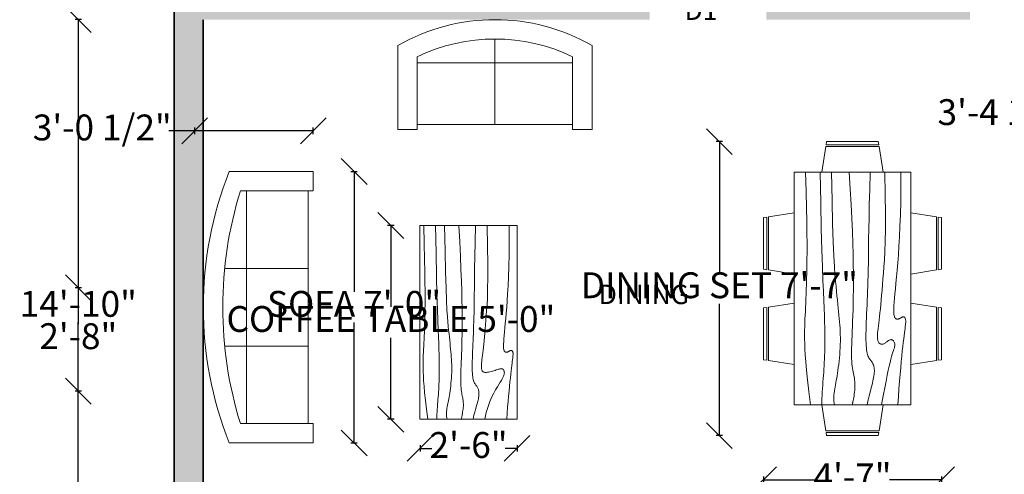
# Model space of a CAD drawing. Units: inches. Extents: x 2530 to 3100, y 543 to 1175.
# Tile 3 of 5: x 2578 to 2883, y 804 to 944. Entities that reach past the tile are written whole.
import ezdxf

# ---------------------------------------------------------------- set-up
doc = ezdxf.new("R2010")
doc.units = ezdxf.units.IN
for name, color, linetype, lineweight in [('A-ANNO-DIMS', 2, 'Continuous', 18), ('A-ANNO-TEXT', 7, 'Continuous', 18), ('A-AREA-IDEN', 7, 'Continuous', 18), ('A-FURN', 8, 'Continuous', 18), ('A-WALL', 7, 'Continuous', 35), ('A-WALL-PATT', 30, 'Continuous', 13)]:
    doc.layers.add(name, color=color, linetype=linetype, lineweight=lineweight)
doc.styles.get("Standard").update_dxf_attribs({"font": 'arial.ttf'})
doc.dimstyles.new('ISO-25', dxfattribs={"dimtxt": 8, "dimasz": 8, "dimexe": 1, "dimexo": 1, "dimtad": 0, "dimtih": 1, "dimtoh": 1, "dimlunit": 3, "dimtxsty": 'Standard', "dimblk": 'OBLIQUE', "dimcen": 2.5, "dimadec": 0, "dimazin": 0, "dimtfac": 1, "dimtmove": 0, "dimatfit": 3, "dimfxl": 1, "dimfxlon": 1, "dimarcsym": 0})

# ---------------------------------------------------------------- blocks, each defined once
blk = doc.blocks.new('Sofa - Roundback 7 ft.')
for p, q in [((-12.00002, -32.4421), (-12.00003, -6.5971)), ((11.99997, -32.4421), (11.99998, -6.5971)), ((-36.000027, -34), (-36.000027, -11.4696)), ((35.99998, -34), (35.99998, -11.4696)), ((-35.999844, -13.3819), (35.9998, -13.3819)), ((-36.000027, -32.4421), (35.99998, -32.4421))]:
    blk.add_line(p, q)
for points in [[(-36.000027, -34), (-42.000027, -34), (-42.000027, -8)], [(41.99998, -8), (41.99998, -34), (35.99998, -34)]]:
    blk.add_lwpolyline(points)
for centre, radius, start, end in [((0, -114.25), 114.25, 68.43141, 111.5686), ((-0.00001, -127.1968), 121.1968, 72.72033, 107.2797)]:
    blk.add_arc(centre, radius, start, end)
blk = doc.blocks.new('Sofa - Roundback Loveseat 5 ft.')
for p, q in [((0, -32.44198), (0, -5.99998)), ((-24, -33.99998), (-24, -11.46958)), ((24.00004, -33.99998), (24.00004, -11.46958)), ((-23.9998, -13.38178), (23.99986, -13.38178)), ((-24, -32.44198), (24.00004, -32.44198))]:
    blk.add_line(p, q)
for points in [[(-24, -33.99998), (-30, -33.99998), (-30, -7.99998)], [(30.00004, -7.99998), (30.00004, -33.99998), (24.00004, -33.99998)]]:
    blk.add_lwpolyline(points)
for centre, radius, start, end in [((0, -60.24998), 60.24998, 60.13715, 119.8628), ((0, -61.38438), 55.38444, 64.32083, 115.6792)]:
    blk.add_arc(centre, radius, start, end)
blk = doc.blocks.new('Dining Set - 36 x 72 in.')
for p, q in [((-22, 27.5), (-22.1562, 26.50042)), ((-22, 27.5), (-6, 27.5)), ((-5.8437, 26.49966), (-6, 27.5)), ((6, 27.5), (5.8438, 26.50042)), ((6, 27.5), (22, 27.5)), ((22.1563, 26.49966), (22, 27.5)), ((-22.2343, 26.00059), (-23.4847, 17.99762)), ((-22.2304, 26), (-5.7608, 26)), ((-5.8416, 26.5), (-22.1534, 26.5)), ((-4.5152, 17.99762), (-5.7655, 25.99926)), ((5.7657, 26.00059), (4.5153, 17.99762)), ((5.7696, 26), (22.2392, 26)), ((22.1584, 26.5), (5.8466, 26.5)), ((23.4848, 17.99762), (22.2345, 25.99926)), ((36, 18), (-36, 18)), ((-36, 18), (-36, -18)), ((36, -18), (36, 18)), ((-44.0006, 8.23428), (-35.9976, 9.48474)), ((44.0006, 8.23428), (35.9976, 9.48474)), ((-45.5, 8), (-44.5004, 8.15617)), ((-45.5, 8), (-45.5, -8)), ((-44.5, -8.15843), (-44.5, 8.15338)), ((-44, 8.23041), (-44, -8.23915)), ((44, 8.23041), (44, -8.23915)), ((44.5, -8.15843), (44.5, 8.15338)), ((45.5, 8), (44.5005, 8.15617)), ((45.5, 8), (45.5, -8)), ((-44.4997, -8.15631), (-45.5, -8)), ((-35.9976, -9.48476), (-43.9993, -8.2345)), ((35.9976, -9.48476), (43.9993, -8.2345)), ((44.4997, -8.15631), (45.5, -8)), ((-36, -18), (36, -18)), ((-22.2343, -26.0006), (-23.4847, -17.99762)), ((-4.5152, -17.99762), (-5.7655, -25.99928)), ((5.7657, -26.0006), (4.5153, -17.99762)), ((23.4848, -17.99762), (22.2345, -25.99928)), ((-22.2304, -26), (-5.7608, -26)), ((-22, -27.5), (-22.1562, -26.50044)), ((-5.8416, -26.5), (-22.1534, -26.5)), ((-5.8437, -26.49967), (-6, -27.5)), ((5.7696, -26), (22.2392, -26)), ((6, -27.5), (5.8438, -26.50044)), ((22.1584, -26.5), (5.8466, -26.5)), ((22.1563, -26.49967), (22, -27.5)), ((-22, -27.5), (-6, -27.5)), ((6, -27.5), (22, -27.5))]:
    blk.add_line(p, q)
for points in [[(-36, 15), (-31.1772, 14.97754), (-26.8079, 14.91406), (-22.8538, 14.81543), (-19.276, 14.6875), (-16.0362, 14.53613), (-13.0957, 14.36718), (-10.4159, 14.18652), (-7.9583, 14), (-5.6904, 13.81315), (-3.6035, 13.63021), (-1.6954, 13.45508), (0.0365, 13.29166), (1.5945, 13.14388), (2.9811, 13.01562), (4.1988, 12.9108), (5.25, 12.83333), (6.1393, 12.78613), (6.8802, 12.76823), (7.4883, 12.77767), (7.9792, 12.8125), (8.3685, 12.87077), (8.6719, 12.95052), (8.9049, 13.0498), (9.0833, 13.16666), (9.2205, 13.29899), (9.3216, 13.44401), (9.3895, 13.59879), (9.4271, 13.76041), (9.4373, 13.92594), (9.4232, 14.09245), (9.3875, 14.257), (9.3333, 14.41666), (9.2638, 14.56917), (9.1836, 14.71484), (9.0975, 14.85465), (9.0104, 14.98958), (8.9272, 15.1206), (8.8529, 15.2487), (8.7922, 15.37483), (8.75, 15.5), (8.7305, 15.62467), (8.7344, 15.74739), (8.7617, 15.86621), (8.8125, 15.97916), (8.8867, 16.08431), (8.9844, 16.17968), (9.1055, 16.26334), (9.25, 16.33333), (9.4189, 16.38802), (9.6172, 16.42708), (9.8506, 16.45052), (10.125, 16.45833), (10.4463, 16.45052), (10.8203, 16.42708), (11.2529, 16.38802), (11.75, 16.33333), (12.3184, 16.26318), (12.9694, 16.17838), (13.7151, 16.07991), (14.5677, 15.96875), (15.5395, 15.84586), (16.6426, 15.71224), (17.8893, 15.56884), (19.2917, 15.41666), (20.859, 15.25667), (22.5879, 15.08984), (24.4721, 14.91715), (26.5052, 14.73958), (28.6809, 14.5581), (30.9929, 14.3737), (33.4347, 14.18733), (36, 14)], [(-36, 10), (-28.9766, 10.14274), (-23.1725, 10.20442), (-18.4241, 10.19775), (-14.5677, 10.13541), (-11.4399, 10.03011), (-8.877, 9.89453), (-6.7154, 9.74137), (-4.7917, 9.58333), (-2.9698, 9.43082), (-1.2246, 9.28515), (0.4415, 9.14534), (2.026, 9.01041), (3.5266, 8.87939), (4.9408, 8.7513), (6.266, 8.62516), (7.5, 8.5), (8.6411, 8.37549), (9.6914, 8.2539), (10.6538, 8.13818), (11.5312, 8.03125), (12.3267, 7.93603), (13.043, 7.85547), (13.6831, 7.79248), (14.25, 7.75), (14.7471, 7.7303), (15.1797, 7.73307), (15.5537, 7.75732), (15.875, 7.80208), (16.1494, 7.86637), (16.3828, 7.94922), (16.5811, 8.04964), (16.75, 8.16666), (16.8944, 8.29915), (17.0143, 8.44531), (17.1089, 8.60319), (17.1771, 8.77083), (17.218, 8.94629), (17.2305, 9.1276), (17.2137, 9.31282), (17.1667, 9.5), (17.0895, 9.6875), (16.987, 9.875), (16.8649, 10.0625), (16.7292, 10.25), (16.5856, 10.4375), (16.4401, 10.625), (16.2985, 10.8125), (16.1667, 11), (16.05, 11.18733), (15.9518, 11.3737), (15.8752, 11.5581), (15.8229, 11.73958), (15.798, 11.91715), (15.8034, 12.08984), (15.842, 12.25667), (15.9167, 12.41666), (16.0295, 12.56836), (16.1784, 12.70833), (16.3605, 12.83268), (16.5729, 12.9375), (16.8127, 13.01888), (17.0768, 13.07291), (17.3625, 13.0957), (17.6667, 13.08333), (17.9894, 13.03312), (18.3418, 12.94726), (18.7382, 12.82918), (19.1927, 12.68229), (19.7195, 12.51001), (20.3327, 12.31575), (21.0465, 12.10294), (21.875, 11.875), (22.8357, 11.63354), (23.959, 11.37304), (25.2786, 11.08618), (26.8282, 10.76562), (28.6414, 10.40405), (30.752, 9.99414), (33.1936, 9.52856), (36, 9)], [(-36, 5.5), (-30.7157, 5.3348), (-26.069, 5.20963), (-21.9946, 5.11767), (-18.4271, 5.05208), (-15.3009, 5.00602), (-12.5508, 4.97265), (-10.1112, 4.94515), (-7.9167, 4.91666), (-5.909, 4.88167), (-4.0586, 4.83984), (-2.3429, 4.79215), (-0.7396, 4.73958), (0.7739, 4.6831), (2.22, 4.6237), (3.6213, 4.56233), (5, 4.5), (6.373, 4.43782), (7.7344, 4.3776), (9.0723, 4.32129), (10.375, 4.27083), (11.6309, 4.22819), (12.8281, 4.19531), (13.9551, 4.17415), (15, 4.16666), (15.954, 4.17448), (16.819, 4.19791), (17.6001, 4.23698), (18.3021, 4.29166), (18.9299, 4.36198), (19.4883, 4.44791), (19.9823, 4.54948), (20.4167, 4.66666), (20.7969, 4.79899), (21.1302, 4.94401), (21.4245, 5.09879), (21.6875, 5.26041), (21.9271, 5.42594), (22.1511, 5.59245), (22.3672, 5.757), (22.5834, 5.91666), (22.8065, 6.06868), (23.0404, 6.21093), (23.2879, 6.34147), (23.5521, 6.45833), (23.8358, 6.55957), (24.142, 6.64323), (24.4735, 6.70735), (24.8334, 6.75), (25.2235, 6.76969), (25.642, 6.76692), (26.0858, 6.74267), (26.5521, 6.69791), (27.0379, 6.63362), (27.5404, 6.55078), (28.0565, 6.45036), (28.5834, 6.33333), (29.1242, 6.19987), (29.7071, 6.04687), (30.3661, 5.87044), (31.1354, 5.66666), (32.0493, 5.43164), (33.142, 5.16146), (34.4475, 4.85221), (36, 4.5)], [(-36, -1), (-30.7915, -0.6591), (-26.0195, -0.38216), (-21.6519, -0.16284), (-17.6563, 0.00521), (-14.0005, 0.12833), (-10.6523, 0.21289), (-7.5796, 0.26522), (-4.75, 0.29166), (-2.134, 0.29793), (0.2878, 0.28711), (2.5317, 0.26163), (4.6146, 0.22396), (6.5529, 0.17651), (8.3633, 0.12174), (10.0623, 0.06209), (11.6667, 0), (13.1899, -0.06201), (14.6341, -0.1211), (15.9982, -0.17432), (17.2813, -0.21875), (18.4823, -0.25147), (19.6003, -0.26953), (20.6343, -0.27002), (21.5834, -0.25), (22.4481, -0.20768), (23.2357, -0.14584), (23.9549, -0.06836), (24.6146, 0.02083), (25.2235, 0.11784), (25.7904, 0.21875), (26.3241, 0.31966), (26.8334, 0.41666), (27.3265, 0.50618), (27.8099, 0.58593), (28.2894, 0.65397), (28.7709, 0.70833), (29.2601, 0.74707), (29.763, 0.76823), (30.2855, 0.76985), (30.8334, 0.75), (31.4088, 0.70784), (31.9994, 0.64713), (32.589, 0.57275), (33.1615, 0.48958), (33.7008, 0.4025), (34.1908, 0.3164), (34.6153, 0.23616), (34.9584, 0.16666), (35.2099, 0.11165), (35.3848, 0.07031), (35.504, 0.04069), (35.5886, 0.02083), (35.6594, 0.00879), (35.7377, 0.0026), (35.8442, 0.00032), (36, 0)], [(-36, -6.5), (-27.1843, -6.31267), (-20.084, -6.1263), (-14.469, -5.9419), (-10.1094, -5.76042), (-6.7752, -5.58285), (-4.2363, -5.41016), (-2.2629, -5.24333), (-0.625, -5.08334), (0.8708, -4.93099), (2.2715, -4.78646), (3.5872, -4.64974), (4.8281, -4.52084), (6.0046, -4.39974), (7.127, -4.28646), (8.2053, -4.18099), (9.25, -4.08334), (10.2705, -3.99382), (11.2734, -3.91407), (12.2647, -3.84603), (13.25, -3.79167), (14.2354, -3.75293), (15.2266, -3.73177), (16.2295, -3.73015), (17.25, -3.75), (18.2912, -3.79248), (19.3451, -3.85547), (20.4009, -3.93604), (21.4479, -4.03125), (22.4754, -4.13819), (23.4727, -4.25391), (24.4289, -4.37549), (25.3334, -4.5), (26.1785, -4.62492), (26.9694, -4.74935), (27.7145, -4.87281), (28.4219, -4.99479), (29.1, -5.11483), (29.7572, -5.23242), (30.4016, -5.34709), (31.0417, -5.45834), (31.6837, -5.56437), (32.3262, -5.65821), (32.9658, -5.73153), (33.599, -5.77604), (34.2224, -5.78345), (34.8327, -5.74545), (35.4264, -5.65373), (36, -5.5)], [(-36, -10), (-26.4022, -9.81299), (-18.4675, -9.62891), (-11.9839, -9.45069), (-6.7396, -9.28125), (-2.5226, -9.12354), (0.8789, -8.98047), (3.6769, -8.85498), (6.0833, -8.75), (8.2767, -8.66765), (10.3021, -8.60677), (12.1712, -8.56543), (13.8958, -8.54167), (15.4876, -8.53353), (16.9583, -8.53907), (18.3197, -8.55632), (19.5834, -8.58334), (20.7616, -8.61841), (21.8685, -8.66081), (22.9188, -8.71004), (23.9271, -8.76563), (24.9081, -8.82707), (25.8763, -8.89388), (26.8465, -8.96558), (27.8334, -9.04167), (28.8474, -9.12118), (29.8828, -9.20117), (30.93, -9.27824), (31.9792, -9.34896), (33.0205, -9.40991), (34.0443, -9.45768), (35.0407, -9.48885), (36, -9.5)], [(-36, -14.5), (-30.0881, -14.33513), (-25.0332, -14.21224), (-20.7312, -14.12647), (-17.0781, -14.07292), (-13.97, -14.04671), (-11.3027, -14.04297), (-8.9724, -14.05681), (-6.875, -14.08334), (-4.9224, -14.11833), (-3.0905, -14.16016), (-1.3709, -14.20785), (0.2448, -14.26042), (1.7647, -14.3169), (3.1973, -14.3763), (4.5507, -14.43767), (5.8333, -14.5), (7.0554, -14.5621), (8.235, -14.62175), (9.3922, -14.67652), (10.5469, -14.72396), (11.7192, -14.76164), (12.929, -14.78711), (14.1965, -14.79794), (15.5417, -14.79167), (16.9933, -14.76424), (18.6152, -14.70508), (20.4804, -14.60197), (22.6615, -14.44271), (25.2312, -14.21509), (28.2624, -13.9069), (31.8277, -13.50594), (36, -13)]]:
    blk.add_lwpolyline(points)
blk = doc.blocks.new('Table - Rectangular Woodgrain 60 x 30 in.')
for p, q in [((0, 0), (0, -30)), ((60, 0), (0, 0)), ((60, -30), (60, 0)), ((0, -30), (60, -30))]:
    blk.add_line(p, q)
for points in [[(0, -2.4), (4.8155, -2.418), (9.0302, -2.4688), (12.709, -2.5477), (15.9167, -2.65), (18.7181, -2.7711), (21.1781, -2.9063), (23.3616, -3.0508), (25.3333, -3.2), (27.1477, -3.3495), (28.8172, -3.4958), (30.3437, -3.636), (31.7291, -3.7667), (32.9756, -3.8849), (34.0849, -3.9875), (35.059, -4.0714), (35.9, -4.1334), (36.6114, -4.1711), (37.2041, -4.1854), (37.6906, -4.1779), (38.0833, -4.15), (38.3948, -4.1034), (38.6375, -4.0396), (38.8239, -3.9602), (38.9666, -3.8667), (39.0764, -3.7608), (39.1573, -3.6448), (39.2116, -3.521), (39.2416, -3.3917), (39.2498, -3.2593), (39.2385, -3.1261), (39.21, -2.9944), (39.1666, -2.8667), (39.111, -2.7447), (39.0468, -2.6281), (38.978, -2.5163), (38.9083, -2.4083), (38.8418, -2.3035), (38.7823, -2.201), (38.7337, -2.1001), (38.7, -2), (38.6844, -1.9003), (38.6875, -1.8021), (38.7094, -1.707), (38.75, -1.6167), (38.8094, -1.5326), (38.8875, -1.4563), (38.9844, -1.3893), (39.1, -1.3333), (39.2351, -1.2896), (39.3937, -1.2583), (39.5804, -1.2396), (39.8, -1.2333), (40.057, -1.2396), (40.3562, -1.2583), (40.7023, -1.2896), (41.1, -1.3333), (41.5547, -1.3895), (42.0755, -1.4573), (42.6721, -1.5361), (43.3542, -1.625), (44.1316, -1.7233), (45.014, -1.8302), (46.0114, -1.9449), (47.1333, -2.0667), (48.3862, -2.1947), (49.7625, -2.3281), (51.2513, -2.4663), (52.8416, -2.6083), (54.5226, -2.7535), (56.2833, -2.9011), (58.1127, -3.0501), (60, -3.2)], [(0, -9.2), (6.5759, -9.0858), (11.9385, -9.0365), (16.2527, -9.0418), (19.6833, -9.0917), (22.3952, -9.1759), (24.5531, -9.2844), (26.322, -9.4069), (27.8666, -9.5333), (29.3241, -9.6553), (30.7203, -9.7719), (32.0532, -9.8837), (33.3208, -9.9917), (34.5213, -10.0965), (35.6526, -10.199), (36.7128, -10.2999), (37.7, -10.4), (38.6129, -10.4996), (39.4531, -10.5969), (40.223, -10.6895), (40.925, -10.775), (41.5613, -10.8512), (42.1344, -10.9156), (42.6465, -10.966), (43.1, -11), (43.4976, -11.0158), (43.8437, -11.0136), (44.143, -10.9942), (44.4, -10.9583), (44.6195, -10.9069), (44.8062, -10.8406), (44.9648, -10.7603), (45.1, -10.6667), (45.2155, -10.5598), (45.3114, -10.4365), (45.3871, -10.2929), (45.4416, -10.125), (45.4743, -9.929), (45.4844, -9.7011), (45.4709, -9.4371), (45.4333, -9.1333), (45.3716, -8.7883), (45.2896, -8.4104), (45.1919, -8.0107), (45.0833, -7.6), (44.9685, -7.1893), (44.8521, -6.7896), (44.7388, -6.4117), (44.6333, -6.0667), (44.54, -5.7628), (44.4614, -5.4979), (44.4001, -5.2675), (44.3583, -5.0667), (44.3384, -4.8909), (44.3427, -4.7354), (44.3736, -4.5956), (44.4333, -4.4667), (44.5236, -4.3453), (44.6427, -4.2333), (44.7884, -4.1339), (44.9583, -4.05), (45.1501, -3.9849), (45.3614, -3.9417), (45.59, -3.9234), (45.8333, -3.9333), (46.0915, -3.9749), (46.3734, -4.0531), (46.6906, -4.1736), (47.0542, -4.3417), (47.4756, -4.5629), (47.9661, -4.8427), (48.5372, -5.1866), (49.2, -5.6), (49.9676, -6.0844), (50.8594, -6.625), (51.8965, -7.2031), (53.1, -7.8), (54.491, -8.3969), (56.0906, -8.975), (57.9199, -9.5156), (60, -10)], [(0, -12.8), (5.1847, -12.9322), (9.6213, -13.0323), (13.3963, -13.1059), (16.5958, -13.1583), (19.3063, -13.1952), (21.614, -13.2219), (23.6054, -13.2439), (25.3666, -13.2667), (26.9728, -13.2947), (28.4531, -13.3281), (29.8256, -13.3663), (31.1083, -13.4083), (32.3191, -13.4535), (33.476, -13.501), (34.597, -13.5501), (35.7, -13.6), (36.7984, -13.6497), (37.8875, -13.6979), (38.9578, -13.743), (40, -13.7833), (41.0047, -13.8174), (41.9625, -13.8438), (42.864, -13.8607), (43.7, -13.8667), (44.4631, -13.8604), (45.1552, -13.8417), (45.7801, -13.8104), (46.3416, -13.7667), (46.8439, -13.7104), (47.2906, -13.6417), (47.6858, -13.5604), (48.0333, -13.4667), (48.3375, -13.3608), (48.6042, -13.2448), (48.8396, -13.121), (49.05, -12.9917), (49.2417, -12.8593), (49.4208, -12.7261), (49.5937, -12.5944), (49.7667, -12.4667), (49.9452, -12.3451), (50.1323, -12.2313), (50.3303, -12.1268), (50.5416, -12.0333), (50.7686, -11.9524), (51.0135, -11.8854), (51.2788, -11.8341), (51.5666, -11.8), (51.8785, -11.7843), (52.2116, -11.7865), (52.562, -11.8059), (52.926, -11.8417), (53.2998, -11.8931), (53.6795, -11.9594), (54.0614, -12.0397), (54.4416, -12.1333), (54.8223, -12.2401), (55.2293, -12.3625), (55.6942, -12.5037), (56.2489, -12.6667), (56.9251, -12.8547), (57.7545, -13.0708), (58.7689, -13.3182), (60, -13.6)], [(0, -18), (5.124, -17.7273), (9.6609, -17.5057), (13.6705, -17.3303), (17.2125, -17.1958), (20.3467, -17.0973), (23.1328, -17.0297), (25.6307, -16.9878), (27.9, -16.9667), (29.9928, -16.9617), (31.9302, -16.9703), (33.7254, -16.9907), (35.3917, -17.0208), (36.9423, -17.0588), (38.3906, -17.1026), (39.7499, -17.1503), (41.0333, -17.2), (42.2519, -17.2496), (43.4073, -17.2969), (44.4986, -17.3395), (45.525, -17.375), (46.4858, -17.4012), (47.3802, -17.4156), (48.2074, -17.416), (48.9667, -17.4), (49.6583, -17.3662), (50.2872, -17.3167), (50.8595, -17.2547), (51.3812, -17.1833), (51.8584, -17.1057), (52.2971, -17.025), (52.7034, -16.9443), (53.0833, -16.8667), (53.443, -16.7951), (53.789, -16.7313), (54.128, -16.6768), (54.4666, -16.6334), (54.8115, -16.6024), (55.1693, -16.5854), (55.5465, -16.5841), (55.95, -16.6), (56.3828, -16.6337), (56.8346, -16.6823), (57.2915, -16.7418), (57.7396, -16.8084), (58.165, -16.878), (58.5539, -16.9469), (58.8924, -17.0111), (59.1666, -17.0667), (59.3679, -17.1107), (59.5078, -17.1438), (59.6032, -17.1675), (59.6708, -17.1833), (59.7275, -17.193), (59.7901, -17.1979), (59.8753, -17.1998), (60, -17.2)], [(0, -22.4), (8.0098, -22.2501), (14.4094, -22.1011), (19.4168, -21.9535), (23.25, -21.8083), (26.1269, -21.6663), (28.2656, -21.5281), (29.884, -21.3947), (31.2, -21.2667), (32.3967, -21.1448), (33.5172, -21.0292), (34.5697, -20.9198), (35.5625, -20.8167), (36.5037, -20.7198), (37.4015, -20.6292), (38.2642, -20.5448), (39.1, -20.4667), (39.9164, -20.3951), (40.7187, -20.3313), (41.5117, -20.2768), (42.3, -20.2333), (43.0883, -20.2024), (43.8812, -20.1854), (44.6836, -20.1841), (45.5, -20.2), (46.3328, -20.234), (47.1747, -20.2844), (48.0163, -20.3488), (48.8479, -20.425), (49.66, -20.5106), (50.4429, -20.6031), (51.1872, -20.7004), (51.8833, -20.8), (52.5246, -20.8999), (53.1166, -20.9995), (53.6681, -21.0983), (54.1875, -21.1958), (54.6834, -21.2919), (55.1646, -21.3859), (55.6394, -21.4777), (56.1167, -21.5667), (56.6028, -21.6515), (57.0961, -21.7266), (57.5929, -21.7852), (58.0896, -21.8208), (58.5823, -21.8268), (59.0674, -21.7964), (59.5412, -21.723), (60, -21.6)], [(0, -25.2), (8.6355, -25.0504), (15.7026, -24.9031), (21.4049, -24.7606), (25.9458, -24.625), (29.529, -24.4988), (32.3578, -24.3844), (34.6359, -24.284), (36.5667, -24.2), (38.3213, -24.1341), (39.9417, -24.0854), (41.437, -24.0523), (42.8167, -24.0333), (44.0901, -24.0268), (45.2667, -24.0313), (46.3557, -24.0451), (47.3667, -24.0667), (48.309, -24.0947), (49.1928, -24.1287), (50.0284, -24.168), (50.826, -24.2125), (51.5959, -24.2617), (52.3483, -24.3151), (53.0935, -24.3725), (53.8417, -24.4334), (54.6009, -24.497), (55.3699, -24.561), (56.1454, -24.6226), (56.9239, -24.6792), (57.7021, -24.7279), (58.4764, -24.7662), (59.2435, -24.7911), (60, -24.8)], [(0, -28.8), (5.6867, -28.6681), (10.45, -28.5698), (14.407, -28.5012), (17.675, -28.4584), (20.3711, -28.4374), (22.6125, -28.4344), (24.5164, -28.4455), (26.2, -28.4667), (27.762, -28.4947), (29.2276, -28.5281), (30.6033, -28.5663), (31.8958, -28.6084), (33.1118, -28.6535), (34.2578, -28.7011), (35.3405, -28.7501), (36.3666, -28.8), (37.3443, -28.8497), (38.288, -28.8974), (39.2137, -28.9412), (40.1375, -28.9792), (41.0753, -29.0093), (42.0432, -29.0297), (43.0572, -29.0384), (44.1333, -29.0333), (45.2936, -29.0114), (46.5843, -28.9641), (48.0579, -28.8816), (49.7666, -28.7542), (51.7629, -28.5721), (54.0989, -28.3255), (56.8272, -28.0048), (60, -27.6)]]:
    blk.add_lwpolyline(points)
blk = doc.blocks.new('_Oblique')
at = {"color": 0, "linetype": 'ByBlock', "lineweight": -2}
blk.add_line((-0.5, -0.5), (0.5, 0.5), dxfattribs=at)
blk = doc.blocks.new('*D38')
at = {"layer": 'A-ANNO-DIMS', "color": 0, "lineweight": -2, "transparency": 16777216}
for p, q in [((2911.92, 791.86), (2903.92, 791.86)), ((2911.92, 790.86), (2911.92, 792.86)), ((2938.56, 791.86), (2911.92, 791.86)), ((2938.56, 790.86), (2938.56, 792.86))]:
    blk.add_line(p, q, dxfattribs=at)
at = {"layer": 'Defpoints', "color": 0, "transparency": 16777216}
for p in [(2911.92, 791.86), (2911.92, 787.87), (2938.56, 787.87)]:
    blk.add_point(p, dxfattribs=at)
at = {"layer": 'A-ANNO-DIMS', "color": 0, "lineweight": -2, "transparency": 16777216, "xscale": 8, "yscale": 8, "zscale": 8, "rotation": 180}
blk.add_blockref('_Oblique', (2911.92, 791.86), dxfattribs=at)
at = {"layer": 'A-ANNO-DIMS', "color": 0, "lineweight": -2, "transparency": 16777216, "xscale": 8, "yscale": 8, "zscale": 8}
blk.add_blockref('_Oblique', (2938.56, 791.86), dxfattribs=at)
at = {"layer": 'A-ANNO-DIMS', "color": 0, "transparency": 16777216, "insert": (2837.6, 791.86), "char_height": 8, "attachment_point": 5}
blk.add_mtext('REFRIGERATOR 2\'-2 1/2"', dxfattribs=at)
blk = doc.blocks.new('*D40')
at = {"layer": 'A-ANNO-DIMS', "color": 0, "lineweight": -2, "transparency": 16777216}
for p, q in [((2680.52, 897.41), (2682.52, 897.41)), ((2681.52, 897.41), (2681.52, 860.17)), ((2681.52, 813.41), (2681.52, 850.64)), ((2680.52, 813.41), (2682.52, 813.41))]:
    blk.add_line(p, q, dxfattribs=at)
at = {"layer": 'Defpoints', "color": 0, "transparency": 16777216}
for p in [(2668.92, 897.41), (2681.52, 897.41), (2668.92, 813.41)]:
    blk.add_point(p, dxfattribs=at)
at = {"layer": 'A-ANNO-DIMS', "color": 0, "lineweight": -2, "transparency": 16777216, "xscale": 8, "yscale": 8, "zscale": 8}
for p, rotation in [((2681.52, 897.41), 90), ((2681.52, 813.41), 270)]:
    blk.add_blockref('_Oblique', p, dxfattribs=dict(at, rotation=rotation))
at = {"layer": 'A-ANNO-DIMS', "color": 0, "transparency": 16777216, "insert": (2681.52, 855.41), "char_height": 8, "attachment_point": 5}
blk.add_mtext('SOFA 7\'-0"', dxfattribs=at)
blk = doc.blocks.new('*D41')
at = {"layer": 'A-ANNO-DIMS', "color": 0, "lineweight": -2, "transparency": 16777216}
for p, q in [((2632.25, 909.01), (2632.25, 911.01)), ((2668.92, 909.01), (2668.92, 911.01)), ((2632.25, 910.01), (2624.25, 910.01)), ((2668.92, 910.01), (2632.25, 910.01))]:
    blk.add_line(p, q, dxfattribs=at)
at = {"layer": 'Defpoints', "color": 0, "transparency": 16777216}
for p in [(2632.25, 910.01), (2632.25, 897.41), (2668.92, 897.41)]:
    blk.add_point(p, dxfattribs=at)
at = {"layer": 'A-ANNO-DIMS', "color": 0, "lineweight": -2, "transparency": 16777216, "xscale": 8, "yscale": 8, "zscale": 8, "rotation": 180}
blk.add_blockref('_Oblique', (2632.25, 910.01), dxfattribs=at)
at = {"layer": 'A-ANNO-DIMS', "color": 0, "lineweight": -2, "transparency": 16777216, "xscale": 8, "yscale": 8, "zscale": 8}
blk.add_blockref('_Oblique', (2668.92, 910.01), dxfattribs=at)
at = {"layer": 'A-ANNO-DIMS', "color": 0, "transparency": 16777216, "insert": (2603.67, 910.01), "char_height": 8, "attachment_point": 5}
blk.add_mtext('3\'-0 1/2"', dxfattribs=at)
blk = doc.blocks.new('*D42')
at = {"layer": 'A-ANNO-DIMS', "color": 0, "lineweight": -2, "transparency": 16777216}
for p, q in [((2795.43, 906.67), (2793.43, 906.67)), ((2794.43, 906.67), (2794.43, 865.93)), ((2794.43, 815.67), (2794.43, 856.41)), ((2795.43, 815.67), (2793.43, 815.67))]:
    blk.add_line(p, q, dxfattribs=at)
at = {"layer": 'Defpoints', "color": 0, "transparency": 16777216}
for p in [(2808.08, 906.67), (2794.43, 815.67), (2808.08, 815.67)]:
    blk.add_point(p, dxfattribs=at)
at = {"layer": 'A-ANNO-DIMS', "color": 0, "lineweight": -2, "transparency": 16777216, "xscale": 8, "yscale": 8, "zscale": 8}
for p, rotation in [((2794.43, 906.67), 90), ((2794.43, 815.67), 270)]:
    blk.add_blockref('_Oblique', p, dxfattribs=dict(at, rotation=rotation))
at = {"layer": 'A-ANNO-DIMS', "color": 0, "transparency": 16777216, "insert": (2794.43, 861.17), "char_height": 8, "attachment_point": 5}
blk.add_mtext('DINING SET 7\'-7"', dxfattribs=at)
blk = doc.blocks.new('*D43')
at = {"layer": 'A-ANNO-DIMS', "color": 0, "lineweight": -2, "transparency": 16777216}
for p, q in [((2808.08, 803.02), (2808.08, 801.02)), ((2808.08, 802.02), (2824.16, 802.02)), ((2863.08, 802.02), (2847, 802.02)), ((2863.08, 803.02), (2863.08, 801.02))]:
    blk.add_line(p, q, dxfattribs=at)
at = {"layer": 'Defpoints', "color": 0, "transparency": 16777216}
for p in [(2808.08, 815.67), (2863.08, 815.67), (2863.08, 802.02)]:
    blk.add_point(p, dxfattribs=at)
at = {"layer": 'A-ANNO-DIMS', "color": 0, "lineweight": -2, "transparency": 16777216, "xscale": 8, "yscale": 8, "zscale": 8, "rotation": 180}
blk.add_blockref('_Oblique', (2808.08, 802.02), dxfattribs=at)
at = {"layer": 'A-ANNO-DIMS', "color": 0, "lineweight": -2, "transparency": 16777216, "xscale": 8, "yscale": 8, "zscale": 8}
blk.add_blockref('_Oblique', (2863.08, 802.02), dxfattribs=at)
at = {"layer": 'A-ANNO-DIMS', "color": 0, "transparency": 16777216, "insert": (2835.58, 802.02), "char_height": 8, "attachment_point": 5}
blk.add_mtext('4\'-7"', dxfattribs=at)
blk = doc.blocks.new('*D44')
at = {"layer": 'A-ANNO-DIMS', "color": 0, "lineweight": -2, "transparency": 16777216}
for p, q in [((2693.9, 880.73), (2691.9, 880.73)), ((2692.9, 880.73), (2692.9, 855.49)), ((2692.9, 820.73), (2692.9, 845.96)), ((2693.9, 820.73), (2691.9, 820.73))]:
    blk.add_line(p, q, dxfattribs=at)
at = {"layer": 'Defpoints', "color": 0, "transparency": 16777216}
for p in [(2701.9, 880.73), (2692.9, 820.73), (2701.9, 820.73)]:
    blk.add_point(p, dxfattribs=at)
at = {"layer": 'A-ANNO-DIMS', "color": 0, "lineweight": -2, "transparency": 16777216, "xscale": 8, "yscale": 8, "zscale": 8}
for p, rotation in [((2692.9, 880.73), 90), ((2692.9, 820.73), 270)]:
    blk.add_blockref('_Oblique', p, dxfattribs=dict(at, rotation=rotation))
at = {"layer": 'A-ANNO-DIMS', "color": 0, "transparency": 16777216, "insert": (2692.9, 850.73), "char_height": 8, "attachment_point": 5}
blk.add_mtext('COFFEE TABLE 5\'-0"', dxfattribs=at)
blk = doc.blocks.new('*D45')
at = {"layer": 'A-ANNO-DIMS', "color": 0, "lineweight": -2, "transparency": 16777216}
for p, q in [((2701.9, 812.73), (2701.9, 810.73)), ((2731.9, 812.73), (2731.9, 810.73)), ((2701.9, 811.73), (2705.57, 811.73)), ((2731.9, 811.73), (2728.22, 811.73))]:
    blk.add_line(p, q, dxfattribs=at)
at = {"layer": 'Defpoints', "color": 0, "transparency": 16777216}
for p in [(2701.9, 820.73), (2731.9, 820.73), (2731.9, 811.73)]:
    blk.add_point(p, dxfattribs=at)
at = {"layer": 'A-ANNO-DIMS', "color": 0, "lineweight": -2, "transparency": 16777216, "xscale": 8, "yscale": 8, "zscale": 8, "rotation": 180}
blk.add_blockref('_Oblique', (2701.9, 811.73), dxfattribs=at)
at = {"layer": 'A-ANNO-DIMS', "color": 0, "lineweight": -2, "transparency": 16777216, "xscale": 8, "yscale": 8, "zscale": 8}
blk.add_blockref('_Oblique', (2731.9, 811.73), dxfattribs=at)
at = {"layer": 'A-ANNO-DIMS', "color": 0, "transparency": 16777216, "insert": (2716.9, 811.73), "char_height": 8, "attachment_point": 5}
blk.add_mtext('2\'-6"', dxfattribs=at)
blk = doc.blocks.new('*D47')
at = {"layer": 'A-ANNO-DIMS', "color": 0, "lineweight": -2, "transparency": 16777216}
for p, q in [((2597.27, 944.41), (2595.27, 944.41)), ((2596.27, 944.41), (2596.27, 860.12)), ((2596.27, 766.41), (2596.27, 850.7)), ((2597.27, 766.41), (2595.27, 766.41))]:
    blk.add_line(p, q, dxfattribs=at)
at = {"layer": 'Defpoints', "color": 0, "transparency": 16777216}
for p in [(2596.27, 944.41), (2634.92, 944.41), (2634.92, 766.41)]:
    blk.add_point(p, dxfattribs=at)
at = {"layer": 'A-ANNO-DIMS', "color": 0, "lineweight": -2, "transparency": 16777216, "xscale": 8, "yscale": 8, "zscale": 8}
for p, rotation in [((2596.27, 944.41), 90), ((2596.27, 766.41), 270)]:
    blk.add_blockref('_Oblique', p, dxfattribs=dict(at, rotation=rotation))
at = {"layer": 'A-ANNO-DIMS', "color": 0, "transparency": 16777216, "insert": (2596.27, 855.41), "char_height": 8, "attachment_point": 5}
blk.add_mtext('14\'-10"', dxfattribs=at)
blk = doc.blocks.new('*D65')
at = {"layer": 'A-ANNO-DIMS', "color": 0, "lineweight": -2, "transparency": 16777216}
for p, q in [((2597.27, 861.41), (2595.27, 861.41)), ((2596.27, 861.41), (2596.27, 850.12)), ((2596.27, 829.41), (2596.27, 840.7)), ((2597.27, 829.41), (2595.27, 829.41))]:
    blk.add_line(p, q, dxfattribs=at)
at = {"layer": 'Defpoints', "color": 0, "transparency": 16777216}
for p in [(2596.27, 861.41), (2907.92, 861.41), (2907.92, 829.41)]:
    blk.add_point(p, dxfattribs=at)
at = {"layer": 'A-ANNO-DIMS', "color": 0, "lineweight": -2, "transparency": 16777216, "xscale": 8, "yscale": 8, "zscale": 8}
for p, rotation in [((2596.27, 861.41), 90), ((2596.27, 829.41), 270)]:
    blk.add_blockref('_Oblique', p, dxfattribs=dict(at, rotation=rotation))
at = {"layer": 'A-ANNO-DIMS', "color": 0, "transparency": 16777216, "insert": (2596.27, 845.41), "char_height": 8, "attachment_point": 5}
blk.add_mtext('2\'-8"', dxfattribs=at)
blk = doc.blocks.new('*D76')
at = {"layer": 'A-ANNO-DIMS', "color": 0, "lineweight": -2, "transparency": 16777216}
for p, q in [((2911.92, 914.76), (2903.92, 914.76)), ((2911.92, 915.76), (2911.92, 913.76)), ((2952.42, 914.76), (2911.92, 914.76)), ((2952.42, 915.76), (2952.42, 913.76))]:
    blk.add_line(p, q, dxfattribs=at)
at = {"layer": 'Defpoints', "color": 0, "transparency": 16777216}
for p in [(2911.92, 944.41), (2952.42, 944.41), (2911.92, 914.76)]:
    blk.add_point(p, dxfattribs=at)
at = {"layer": 'A-ANNO-DIMS', "color": 0, "lineweight": -2, "transparency": 16777216, "xscale": 8, "yscale": 8, "zscale": 8}
for p, rotation in [((2911.92, 914.76), 180.000000000001), ((2952.42, 914.76), 1.0392e-12)]:
    blk.add_blockref('_Oblique', p, dxfattribs=dict(at, rotation=rotation))
at = {"layer": 'A-ANNO-DIMS', "color": 0, "transparency": 16777216, "insert": (2883.34, 914.76), "char_height": 8, "attachment_point": 5}
blk.add_mtext('3\'-4 1/2"', dxfattribs=at)

msp = doc.modelspace()

# ---------------------------------------------------------------- hatches: boundary and pattern name
at = {"layer": 'A-WALL-PATT'}
h = msp.add_hatch(color=256, dxfattribs=at)
h.dxf.hatch_style = 1
h.paths.add_polyline_path([(2676.945, 1133.407), (2625.918, 1133.407), (2625.918, 584.407), (2673.585, 584.407), (2673.585, 593.407), (2634.918, 593.407), (2634.918, 757.407), (2717.918, 757.407), (2717.918, 766.407), (2634.918, 766.407), (2634.918, 944.407), (2772.918, 944.407), (2772.918, 948.407), (2634.918, 948.407), (2634.918, 1124.407), (2676.945, 1124.407)])
h.paths.add_polyline_path([(2822.346, 1133.407), (2739.946, 1133.407), (2739.946, 1124.407), (2808.918, 1124.407), (2808.918, 1070.407), (2812.918, 1070.407), (2812.918, 1124.407), (2822.346, 1124.407)])
h.paths.add_polyline_path([(2939.91, 1133.407), (2855.561, 1133.407), (2855.561, 1124.407), (2867.918, 1124.407), (2867.918, 1038.407), (2808.918, 1038.407), (2808.918, 944.407), (2871.918, 944.407), (2871.918, 1002.407), (2867.918, 1002.407), (2867.918, 948.407), (2812.918, 948.407), (2812.918, 1034.407), (2871.918, 1034.407), (2871.918, 1124.407), (2939.91, 1124.407)])
h.paths.add_polyline_path([(3054.918, 1133.407), (2997.969, 1133.407), (2997.969, 1124.407), (3045.918, 1124.407), (3045.918, 948.407), (2907.918, 948.407), (2907.918, 928.407), (2911.918, 928.407), (2911.918, 944.407), (2952.418, 944.407), (2952.418, 872.407), (2911.918, 872.407), (2911.918, 888.407), (2907.918, 888.407), (2907.918, 861.407), (2911.918, 861.407), (2911.918, 867.407), (2956.918, 867.407), (2956.918, 944.407), (3045.918, 944.407), (3045.918, 872.407), (2988.918, 872.407), (2988.918, 867.407), (3045.918, 867.407), (3045.918, 766.407), (2986.918, 766.407), (2986.918, 757.407), (3045.918, 757.407), (3045.918, 593.407), (2906.263, 593.407), (2906.263, 584.407), (3054.918, 584.407)])
h.paths.add_polyline_path([(2780.418, 593.407), (2762.418, 593.407), (2762.418, 693.907), (2757.918, 693.907), (2757.918, 593.407), (2719.35, 593.407), (2719.35, 584.407), (2780.418, 584.407)])
h.paths.add_polyline_path([(2846.356, 593.407), (2826.918, 593.407), (2826.918, 757.407), (2826.918, 766.407), (2822.418, 766.407), (2822.418, 693.907), (2794.418, 693.907), (2794.418, 689.407), (2822.418, 689.407), (2822.418, 593.407), (2804.418, 593.407), (2804.418, 584.407), (2846.356, 584.407)])
h.paths.add_polyline_path([(2938.918, 766.407), (2911.918, 766.407), (2911.918, 829.407), (2907.918, 829.407), (2907.918, 766.407), (2886.918, 766.407), (2886.918, 757.407), (2938.918, 757.407)])
h.paths.add_polyline_path([(2822.418, 766.407), (2757.918, 766.407), (2757.918, 757.407), (2757.918, 721.407), (2762.418, 721.407), (2762.418, 757.407), (2822.418, 757.407)])

# ---------------------------------------------------------------- linework, layer by layer
at = {"layer": 'A-WALL'}
for p, q in [((2625.918, 1133.407), (2625.918, 584.407)), ((2634.918, 944.407), (2634.918, 766.407))]:
    msp.add_line(p, q, dxfattribs=at)

# ---------------------------------------------------------------- block references
at = {"layer": 'A-FURN'}
msp.add_blockref('Sofa - Roundback Loveseat 5 ft.', (2725.07, 944.407), dxfattribs=at)
for name, p, rotation in [('Dining Set - 36 x 72 in.', (2835.578, 861.172), 270), ('Sofa - Roundback 7 ft.', (2634.918, 855.407), 90), ('Table - Rectangular Woodgrain 60 x 30 in.', (2731.896, 880.729), 270)]:
    msp.add_blockref(name, p, dxfattribs=dict(at, rotation=rotation))

# ---------------------------------------------------------------- texts
at = {"layer": 'A-ANNO-TEXT', "insert": (2779.529, 950.326), "char_height": 6, "attachment_point": 1}
msp.add_mtext_dynamic_manual_height_columns('\\pxqc;D1', width=18.48176, gutter_width=12.5, heights=[0], dxfattribs=at)
at = {"layer": 'A-AREA-IDEN', "insert": (2747.246, 862.38), "char_height": 6, "attachment_point": 1}
msp.add_mtext_dynamic_manual_height_columns('\\pxqc;DINING', width=47.65744, gutter_width=12.5, heights=[0], dxfattribs=at)

# ---------------------------------------------------------------- dimensions: what is measured, and where the dimension line sits
at = {"layer": 'A-ANNO-DIMS'}
for base, p1, p2, angle, picture, middle in [((2596.268, 944.407), (2634.918, 766.407), (2634.918, 944.407), 90, '*D47', (2596.268, 855.407)), ((2911.918, 914.757), (2952.418, 944.407), (2911.918, 944.407), 180, '*D76', (2883.342, 914.757)), ((2632.251, 910.007), (2668.918, 897.407), (2632.251, 897.407), 180, '*D41', (2603.675, 910.007)), ((2596.268, 861.407), (2907.918, 829.407), (2907.918, 861.407), 90, '*D65', (2596.268, 845.407))]:
    dim = msp.add_linear_dim(base=base, p1=p1, p2=p2, angle=angle, dimstyle='ISO-25', override={"dimdec": 1, "dimlfac": 1, "dimrnd": 0, "dimzin": 1, "dimdsep": 46, "dimlunit": 4, "dimfrac": 2}, dxfattribs=at)
    dim.commit()
    dim.dimension.update_dxf_attribs({"geometry": picture, "text_midpoint": middle})
for base, p1, p2, angle, text, picture, middle in [((2794.428, 815.672), (2808.078, 906.672), (2808.078, 815.672), 270, 'DINING SET <>', '*D42', (2794.428, 861.172)), ((2681.518, 897.407), (2668.918, 813.407), (2668.918, 897.407), 90, 'SOFA <>', '*D40', (2681.518, 855.407)), ((2692.896, 820.729), (2701.896, 880.729), (2701.896, 820.729), 270, 'COFFEE TABLE <>', '*D44', (2692.896, 850.729)), ((2911.918, 791.864), (2938.558, 787.868), (2911.918, 787.868), 180, 'REFRIGERATOR <>', '*D38', (2837.598, 791.864))]:
    dim = msp.add_linear_dim(base=base, p1=p1, p2=p2, angle=angle, text=text, dimstyle='ISO-25', override={"dimdec": 1, "dimlfac": 1, "dimrnd": 0, "dimzin": 1, "dimdsep": 46, "dimlunit": 4, "dimfrac": 2}, dxfattribs=at)
    dim.commit()
    dim.dimension.update_dxf_attribs({"geometry": picture, "text_midpoint": middle})
for base, p1, p2, picture, middle in [((2731.896, 811.729), (2701.896, 820.729), (2731.896, 820.729), '*D45', (2716.896, 811.729)), ((2863.078, 802.022), (2808.078, 815.672), (2863.078, 815.672), '*D43', (2835.578, 802.022))]:
    dim = msp.add_linear_dim(base=base, p1=p1, p2=p2, dimstyle='ISO-25', override={"dimdec": 1, "dimlfac": 1, "dimrnd": 0, "dimzin": 1, "dimdsep": 46, "dimlunit": 4, "dimfrac": 2}, dxfattribs=at)
    dim.commit()
    dim.dimension.update_dxf_attribs({"geometry": picture, "text_midpoint": middle})

doc.saveas('drawing.dxf')
